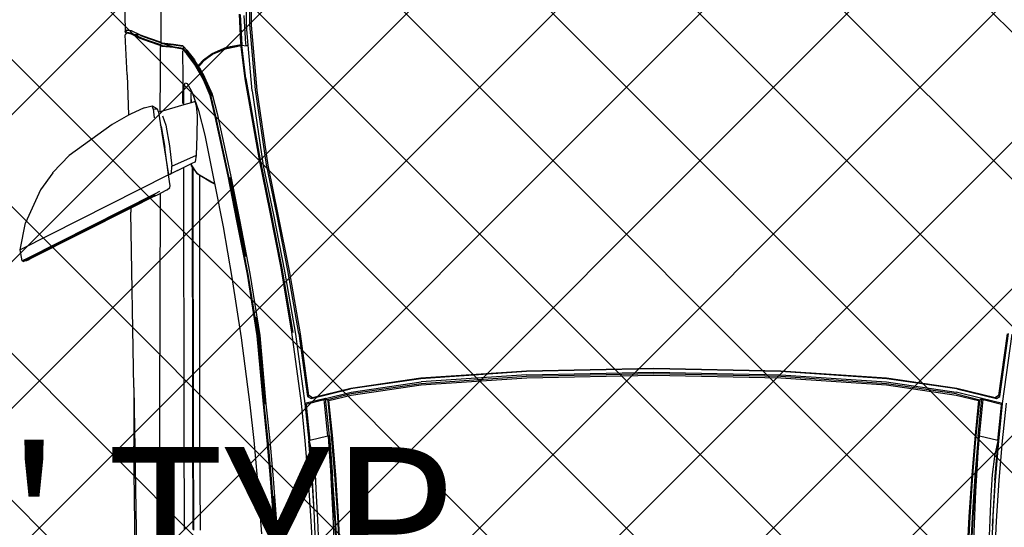
# Model space of a CAD drawing. Units: inches. Extents: x 2167 to 2589, y 1680 to 2489.
# Tile 9 of 38: x 2251 to 2299, y 1771 to 1796. Entities that reach past the tile are written whole.
import ezdxf

# ---------------------------------------------------------------- set-up
doc = ezdxf.new("R2010")
doc.units = ezdxf.units.IN
doc.header["$MEASUREMENT"] = 0
doc.layers.get('0').update_dxf_attribs({"color": 250})
for name, color, linetype, lineweight in [('A-ANNO-DIMS', 2, 'Continuous', 18), ('C-PRKG-VEHS', 8, 'Continuous', 13), ('L-PVMT-PATT', 252, 'Continuous', 13)]:
    doc.layers.add(name, color=color, linetype=linetype, lineweight=lineweight)
doc.layers.add('Edges', color=250, linetype='Continuous')
doc.styles.get("Standard").update_dxf_attribs({"font": 'arial.ttf'})
doc.dimstyles.get("Standard").update_dxf_attribs({"dimtxt": 7, "dimasz": 0.18, "dimexe": 0.18, "dimexo": 0.0625, "dimgap": 0.09, "dimtad": 0, "dimtih": 1, "dimtoh": 1, "dimdec": 1, "dimzin": 0, "dimdsep": 46, "dimlunit": 3, "dimtxsty": 'Standard', "dimcen": 0.09, "dimadec": 0, "dimazin": 0, "dimtfac": 1, "dimtdec": 1, "dimtofl": 0, "dimtmove": 0, "dimatfit": 3, "dimfxl": 1, "dimtolj": 1, "dimtzin": 0, "dimarcsym": 0})

# ---------------------------------------------------------------- blocks, each defined once
blk = doc.blocks.new('Nissan Qashqai pl')
at = {"layer": 'Edges'}
for p, q in [((9.2669, 12.5088), (9.1605, 12.5233)), ((9.1612, 12.5208), (9.2656, 12.5065)), ((9.2789, 12.5131), (9.1617, 12.5292)), ((9.2783, 12.5191), (9.3422, 12.5126)), ((9.2694, 12.5006), (9.2535, 12.4354)), ((9.2543, 12.4356), (9.2707, 12.5028)), ((9.2656, 12.5065), (9.2669, 12.5088)), ((9.2656, 12.5065), (9.2694, 12.5006)), ((9.2707, 12.5028), (9.2669, 12.5088)), ((9.2707, 12.5028), (9.2694, 12.5006)), ((9.2789, 12.5131), (9.2704, 12.4783)), ((9.2724, 12.4804), (9.2799, 12.5114)), ((9.2799, 12.5114), (9.2789, 12.5131)), ((9.3427, 12.5066), (9.2789, 12.5131)), ((9.2819, 12.5112), (9.2799, 12.5114)), ((9.2803, 12.5116), (9.2822, 12.5118)), ((9.3418, 12.5051), (9.2819, 12.5112)), ((9.3418, 12.5051), (9.3346, 12.4741)), ((9.342, 12.5059), (9.3418, 12.5051)), ((9.3687, 12.5), (9.342, 12.5059)), ((9.4087, 12.5003), (9.342, 12.5059)), ((9.3422, 12.5126), (9.4088, 12.507)), ((9.4093, 12.5011), (9.3427, 12.5066)), ((9.3992, 12.496), (9.3687, 12.5)), ((9.4087, 12.5003), (9.4688, 12.4968)), ((9.4088, 12.507), (9.4782, 12.5024)), ((9.4785, 12.4965), (9.4093, 12.5011)), ((9.4688, 12.4968), (9.4789, 12.4964)), ((9.4782, 12.5024), (9.5503, 12.4987)), ((9.2724, 12.4804), (9.2704, 12.4783)), ((9.3346, 12.4741), (9.2724, 12.4804)), ((9.4347, 12.494), (9.3992, 12.496)), ((9.4761, 12.4919), (9.4347, 12.494)), ((9.5168, 12.4903), (9.4761, 12.4919)), ((9.4789, 12.4964), (9.4785, 12.4965)), ((9.4862, 12.4961), (9.4785, 12.4965)), ((9.4789, 12.4964), (9.4862, 12.4961)), ((9.4862, 12.4961), (9.514, 12.4949)), ((9.2704, 12.4783), (9.2598, 12.4348)), ((9.2629, 12.435), (9.2726, 12.4746)), ((9.2649, 12.4348), (9.2741, 12.4725)), ((9.2726, 12.4746), (9.2704, 12.4783)), ((9.3346, 12.4718), (9.2704, 12.4783)), ((9.2746, 12.4744), (9.2726, 12.4746)), ((9.2741, 12.4725), (9.3326, 12.4666)), ((9.333, 12.4685), (9.2746, 12.4744)), ((9.3326, 12.4666), (9.4, 12.4609)), ((9.4004, 12.4629), (9.333, 12.4685)), ((9.3346, 12.4741), (9.3344, 12.4733)), ((9.3344, 12.4733), (9.4017, 12.4677)), ((9.3344, 12.4733), (9.3611, 12.4715)), ((9.3346, 12.4718), (9.4018, 12.4661)), ((9.3611, 12.4715), (9.3918, 12.4695)), ((9.3918, 12.4695), (9.4276, 12.4674)), ((9.4017, 12.4677), (9.472, 12.463)), ((9.4018, 12.4661), (9.472, 12.4614)), ((9.4276, 12.4674), (9.4694, 12.4654)), ((9.4694, 12.4654), (9.5105, 12.4637)), ((9.4, 12.4609), (9.4706, 12.4561)), ((9.4709, 12.4581), (9.4004, 12.4629)), ((9.4706, 12.4561), (9.5443, 12.4522)), ((9.5446, 12.4542), (9.4709, 12.4581)), ((9.472, 12.463), (9.5454, 12.4591)), ((9.472, 12.4614), (9.5454, 12.4576)), ((9.2535, 12.4354), (9.2362, 12.3167)), ((9.2543, 12.4356), (9.2371, 12.3169)), ((9.2426, 12.3164), (9.2598, 12.4348)), ((9.2629, 12.435), (9.2457, 12.3164)), ((9.2476, 12.3163), (9.2649, 12.4348)), ((9.2362, 12.3167), (9.2241, 12.1376)), ((9.2371, 12.3169), (9.2249, 12.1376)), ((9.2305, 12.1375), (9.2426, 12.3164)), ((9.2457, 12.3164), (9.2335, 12.1374)), ((9.2355, 12.1374), (9.2476, 12.3163)), ((9.2241, 12.1376), (9.2195, 11.9221)), ((9.2249, 12.1376), (9.2203, 11.9221)), ((9.2259, 11.9221), (9.2305, 12.1375)), ((9.2335, 12.1374), (9.2289, 11.9221)), ((9.2308, 11.9221), (9.2355, 12.1374)), ((9.2195, 11.9221), (9.2241, 11.7066)), ((9.2203, 11.9221), (9.2249, 11.7065)), ((9.2305, 11.7067), (9.2259, 11.9221)), ((9.2289, 11.9221), (9.2335, 11.7067)), ((9.2355, 11.7068), (9.2308, 11.9221)), ((9.2241, 11.7066), (9.2362, 11.5274)), ((9.2249, 11.7065), (9.2371, 11.5273)), ((9.2305, 11.7067), (9.2426, 11.5277)), ((9.2335, 11.7067), (9.2457, 11.5277)), ((9.2476, 11.5278), (9.2355, 11.7068)), ((9.2362, 11.5274), (9.2535, 11.4087)), ((9.2371, 11.5273), (9.2543, 11.4085)), ((9.2598, 11.4093), (9.2426, 11.5277)), ((9.2457, 11.5277), (9.2629, 11.4092)), ((9.2649, 11.4094), (9.2476, 11.5278)), ((9.2535, 11.4087), (9.2694, 11.3436)), ((9.2707, 11.3414), (9.2543, 11.4085)), ((9.2704, 11.3659), (9.2598, 11.4093)), ((9.2629, 11.4092), (9.2726, 11.3695)), ((9.2741, 11.3716), (9.2649, 11.4094)), ((9.4, 11.3832), (9.3326, 11.3776)), ((9.333, 11.3757), (9.4004, 11.3813)), ((9.4706, 11.388), (9.4, 11.3832)), ((9.4004, 11.3813), (9.4709, 11.3861)), ((9.472, 11.3812), (9.4017, 11.3765)), ((9.472, 11.3828), (9.4018, 11.378)), ((9.4694, 11.3788), (9.4276, 11.3767)), ((9.5105, 11.3805), (9.4694, 11.3788)), ((9.5443, 11.3919), (9.4706, 11.388)), ((9.4709, 11.3861), (9.5446, 11.39)), ((9.5454, 11.3866), (9.472, 11.3828)), ((9.472, 11.3812), (9.5454, 11.3851)), ((9.3346, 11.3724), (9.2704, 11.3659)), ((9.2704, 11.3659), (9.2726, 11.3695)), ((9.2704, 11.3659), (9.2724, 11.3637)), ((9.2704, 11.3659), (9.2789, 11.331)), ((9.3346, 11.37), (9.2724, 11.3637)), ((9.2799, 11.3328), (9.2724, 11.3637)), ((9.2726, 11.3695), (9.2746, 11.3697)), ((9.3326, 11.3776), (9.2741, 11.3716)), ((9.2746, 11.3697), (9.333, 11.3757)), ((9.4017, 11.3765), (9.3344, 11.3708)), ((9.3611, 11.3727), (9.3344, 11.3708)), ((9.3344, 11.3708), (9.3346, 11.37)), ((9.3346, 11.3724), (9.4018, 11.378)), ((9.3346, 11.37), (9.3418, 11.3391)), ((9.3918, 11.3747), (9.3611, 11.3727)), ((9.4276, 11.3767), (9.3918, 11.3747)), ((9.3687, 11.3441), (9.3992, 11.3482)), ((9.3992, 11.3482), (9.4347, 11.3502)), ((9.4605, 11.3465), (9.4087, 11.3438)), ((9.4605, 11.3465), (9.4093, 11.3431)), ((9.4347, 11.3502), (9.4761, 11.3522)), ((9.514, 11.3492), (9.4605, 11.3465)), ((9.4761, 11.3522), (9.5168, 11.3539)), ((9.5503, 11.3455), (9.4782, 11.3418)), ((9.1605, 11.3208), (9.2669, 11.3354)), ((9.2656, 11.3376), (9.1612, 11.3233)), ((9.1617, 11.315), (9.2789, 11.331)), ((9.2694, 11.3436), (9.2656, 11.3376)), ((9.2669, 11.3354), (9.2656, 11.3376)), ((9.2669, 11.3354), (9.2707, 11.3414)), ((9.2694, 11.3436), (9.2707, 11.3414)), ((9.3422, 11.3316), (9.2783, 11.3251)), ((9.2789, 11.331), (9.3427, 11.3375)), ((9.2789, 11.331), (9.2799, 11.3327)), ((9.2799, 11.3328), (9.2819, 11.333)), ((9.2799, 11.3327), (9.2799, 11.3328)), ((9.2799, 11.3327), (9.2811, 11.3325)), ((9.2819, 11.333), (9.3418, 11.3391)), ((9.3418, 11.3391), (9.342, 11.3383)), ((9.342, 11.3383), (9.3687, 11.3441)), ((9.342, 11.3383), (9.4087, 11.3438)), ((9.4088, 11.3371), (9.3422, 11.3316)), ((9.4093, 11.3431), (9.3427, 11.3375)), ((9.4782, 11.3418), (9.4088, 11.3371)), ((9.1605, 11.3208), (9.0538, 11.3023)), ((9.1612, 11.3233), (9.0546, 11.3048)), ((9.0552, 11.2965), (9.1617, 11.315)), ((9.2783, 11.3251), (9.1584, 11.3091)), ((9.0538, 11.3023), (8.9583, 11.2833)), ((9.0546, 11.3048), (8.9591, 11.2859)), ((8.9598, 11.2775), (9.0552, 11.2965)), ((9.1584, 11.3091), (9.0495, 11.2906)), ((9.0497, 11.2918), (9.1586, 11.3104)), ((8.9583, 11.2833), (8.8745, 11.266)), ((8.9591, 11.2859), (8.8754, 11.2687)), ((9.0495, 11.2906), (8.9521, 11.2715)), ((8.9522, 11.2728), (9.0497, 11.2918)), ((9.4736, 11.2793), (9.4063, 11.2743)), ((9.4064, 11.277), (9.4739, 11.282)), ((9.4727, 11.2808), (9.4362, 11.278)), ((9.4727, 11.2808), (9.4732, 11.2808)), ((9.5437, 11.2822), (9.4735, 11.2779)), ((9.5438, 11.2836), (9.4736, 11.2793)), ((9.4739, 11.282), (9.5443, 11.2863)), ((8.8745, 11.266), (8.7481, 11.2473)), ((8.8754, 11.2687), (8.7491, 11.2501)), ((8.8666, 11.2554), (8.9522, 11.2728)), ((8.9521, 11.2715), (8.8666, 11.2541)), ((8.8761, 11.2602), (8.9598, 11.2775)), ((9.1639, 11.2546), (9.2801, 11.2648)), ((9.2804, 11.262), (9.1645, 11.2518)), ((9.2804, 11.2635), (9.1668, 11.2533)), ((9.2801, 11.2648), (9.3418, 11.2713)), ((9.3418, 11.2671), (9.2803, 11.2606)), ((9.3419, 11.2685), (9.2804, 11.262)), ((9.3418, 11.2713), (9.4064, 11.277)), ((9.4062, 11.2729), (9.3418, 11.2671)), ((9.4063, 11.2743), (9.3419, 11.2685)), ((9.4735, 11.2779), (9.4062, 11.2729)), ((8.7481, 11.2473), (8.6375, 11.2376)), ((8.7491, 11.2501), (8.6386, 11.2404)), ((8.7287, 11.2307), (8.8666, 11.2554)), ((8.8666, 11.2541), (8.7292, 11.2295)), ((8.7496, 11.2416), (8.8761, 11.2602)), ((9.0591, 11.2377), (9.1639, 11.2546)), ((9.1644, 11.2503), (9.06, 11.2335)), ((9.1645, 11.2518), (9.0601, 11.235)), ((9.133, 11.2481), (9.1647, 11.2532)), ((9.2803, 11.2606), (9.1644, 11.2503)), ((9.1647, 11.2532), (9.1668, 11.2533)), ((9.3416, 11.2442), (9.4048, 11.2501)), ((9.4048, 11.2501), (9.471, 11.2554)), ((9.471, 11.2554), (9.4997, 11.2573)), ((8.6375, 11.2376), (8.5531, 11.2387)), ((8.6386, 11.2404), (8.5544, 11.2416)), ((8.6387, 11.2319), (8.555, 11.233)), ((8.6699, 11.231), (8.622, 11.228)), ((8.6721, 11.2348), (8.6387, 11.2319)), ((8.6721, 11.2312), (8.6699, 11.231)), ((8.7496, 11.2416), (8.6721, 11.2348)), ((8.6721, 11.2348), (8.6733, 11.2313)), ((8.6721, 11.2312), (8.6721, 11.2318)), ((8.6721, 11.2241), (8.6733, 11.2313)), ((8.6733, 11.2313), (8.6721, 11.2312)), ((8.7287, 11.2307), (8.6721, 11.2241)), ((8.7292, 11.2295), (8.6753, 11.2232)), ((9.0601, 11.235), (8.8941, 11.2023)), ((8.9679, 11.2201), (9.0591, 11.2377)), ((9.06, 11.2335), (8.9696, 11.2157)), ((8.9708, 11.2185), (9.03, 11.2304)), ((9.1676, 11.2229), (9.2814, 11.2377)), ((9.2814, 11.2377), (9.3416, 11.2442)), ((8.6683, 11.2226), (8.6197, 11.2201)), ((8.6203, 11.2213), (8.6721, 11.2241)), ((8.671, 11.2227), (8.6683, 11.2226)), ((8.6721, 11.2241), (8.671, 11.2227)), ((8.6716, 11.2199), (8.671, 11.2227)), ((8.6759, 11.1982), (8.6716, 11.2199)), ((8.6721, 11.2241), (8.6727, 11.2229)), ((8.6772, 11.1988), (8.6721, 11.2241)), ((8.6753, 11.2232), (8.6727, 11.2229)), ((8.6777, 11.1984), (8.6727, 11.2229)), ((8.8918, 11.205), (8.9679, 11.2201)), ((8.9696, 11.2157), (8.8942, 11.2009)), ((8.9318, 11.211), (8.9704, 11.2185)), ((8.9704, 11.2185), (8.9708, 11.2185)), ((9.0656, 11.207), (9.1676, 11.2229)), ((8.6864, 11.1736), (8.6759, 11.1982)), ((8.6875, 11.1744), (8.6772, 11.1988)), ((8.6777, 11.1984), (8.6883, 11.1737)), ((8.7881, 11.1821), (8.8918, 11.205)), ((8.8941, 11.2023), (8.7925, 11.1802)), ((8.8942, 11.2009), (8.7931, 11.1789)), ((8.8961, 11.204), (8.9318, 11.211)), ((8.9797, 11.1924), (9.0656, 11.207)), ((8.7931, 11.1789), (8.7574, 11.1704)), ((8.7575, 11.1744), (8.7881, 11.1821)), ((8.7925, 11.1802), (8.7591, 11.1723)), ((8.9087, 11.1783), (8.9797, 11.1924)), ((8.697, 11.1592), (8.6864, 11.1736)), ((8.6979, 11.1603), (8.6875, 11.1744)), ((8.6883, 11.1737), (8.6987, 11.1597)), ((8.7075, 11.1487), (8.7346, 11.1636)), ((8.7508, 11.1722), (8.7257, 11.1609)), ((8.7529, 11.17), (8.7302, 11.1602)), ((8.7574, 11.1704), (8.7312, 11.1591)), ((8.7346, 11.1636), (8.7577, 11.1732)), ((8.7346, 11.1636), (8.7491, 11.1703)), ((8.7491, 11.1703), (8.7576, 11.1743)), ((8.7508, 11.1722), (8.7491, 11.1703)), ((8.7532, 11.1733), (8.7508, 11.1722)), ((8.7529, 11.17), (8.7577, 11.1732)), ((8.757, 11.1718), (8.7529, 11.17)), ((8.7532, 11.1733), (8.7575, 11.1744)), ((8.7587, 11.1722), (8.757, 11.1718)), ((8.7575, 11.1744), (8.7576, 11.1743)), ((8.7576, 11.1743), (8.7582, 11.1734)), ((8.7577, 11.1732), (8.7582, 11.1734)), ((8.7582, 11.1734), (8.759, 11.1725)), ((8.759, 11.1725), (8.7587, 11.1722)), ((8.7591, 11.1723), (8.7587, 11.1722)), ((8.759, 11.1725), (8.7591, 11.1723)), ((8.8245, 11.1613), (8.9063, 11.1779)), ((8.8893, 11.1486), (8.9021, 11.1697)), ((8.9041, 11.1717), (8.8927, 11.1528)), ((8.9021, 11.1697), (8.9063, 11.1779)), ((8.9075, 11.1781), (8.9041, 11.1717)), ((8.9063, 11.1779), (8.9075, 11.1781)), ((8.9075, 11.1781), (8.9087, 11.1783)), ((8.6917, 11.1371), (8.7075, 11.1487)), ((8.7055, 11.1514), (8.697, 11.1592)), ((8.6987, 11.1596), (8.6979, 11.1603)), ((8.7071, 11.15), (8.6981, 11.1446)), ((8.6987, 11.1597), (8.6988, 11.1596)), ((8.6987, 11.1596), (8.6988, 11.1596)), ((8.6996, 11.1588), (8.6987, 11.1596)), ((8.6988, 11.1596), (8.6996, 11.1588)), ((8.6996, 11.1588), (8.6996, 11.1588)), ((8.7062, 11.1527), (8.6996, 11.1588)), ((8.6996, 11.1588), (8.7062, 11.1527)), ((8.7302, 11.1602), (8.7032, 11.145)), ((8.7312, 11.1591), (8.7042, 11.144)), ((8.707, 11.15), (8.7055, 11.1514)), ((8.7067, 11.1522), (8.7062, 11.1527)), ((8.7083, 11.1508), (8.7067, 11.1522)), ((8.707, 11.15), (8.7083, 11.1508)), ((8.7071, 11.15), (8.707, 11.15)), ((8.707, 11.15), (8.707, 11.15)), ((8.7083, 11.1508), (8.7071, 11.15)), ((8.7083, 11.1507), (8.7102, 11.1519)), ((8.7083, 11.1508), (8.7083, 11.1507)), ((8.7102, 11.1519), (8.7108, 11.1523)), ((8.7108, 11.1523), (8.7257, 11.1609)), ((8.7108, 11.1523), (8.7248, 11.1605)), ((8.7248, 11.1605), (8.7257, 11.1609)), ((8.7524, 11.1401), (8.7828, 11.1508)), ((8.7748, 11.1475), (8.7678, 11.1453)), ((8.7678, 11.1453), (8.7698, 11.1385)), ((8.7916, 11.1488), (8.7748, 11.1475)), ((8.7828, 11.1508), (8.8245, 11.1613)), ((8.8259, 11.1483), (8.7916, 11.1488)), ((8.8585, 11.1473), (8.8259, 11.1483)), ((8.87, 11.1455), (8.8585, 11.1473)), ((8.8771, 11.1054), (8.8585, 11.1473)), ((8.87, 11.1455), (8.8734, 11.1385)), ((8.8893, 11.1486), (8.8751, 11.1387)), ((8.881, 11.1418), (8.8893, 11.1486)), ((8.8913, 11.1506), (8.8893, 11.1486)), ((8.8927, 11.1528), (8.8913, 11.1506)), ((9.3225, 11.1531), (8.8927, 11.1528)), ((9.4936, 11.1538), (9.3225, 11.1531)), ((8.6805, 11.1309), (8.6746, 11.1253)), ((8.687, 11.131), (8.6788, 11.1237)), ((8.6805, 11.1309), (8.6884, 11.1371)), ((8.6815, 11.128), (8.6818, 11.1288)), ((8.6859, 11.132), (8.6817, 11.1282)), ((8.6817, 11.1282), (8.6818, 11.1288)), ((8.6818, 11.1288), (8.6902, 11.136)), ((8.6927, 11.1371), (8.6859, 11.132)), ((8.7042, 11.144), (8.687, 11.131)), ((8.6884, 11.1371), (8.6973, 11.144)), ((8.6884, 11.1371), (8.6917, 11.1371)), ((8.6902, 11.136), (8.6917, 11.1371)), ((8.6923, 11.1371), (8.6927, 11.1371)), ((8.7032, 11.145), (8.6927, 11.1371)), ((8.6973, 11.144), (8.698, 11.1446)), ((8.698, 11.1446), (8.6981, 11.1446)), ((8.7361, 11.1283), (8.7373, 11.1314)), ((8.7373, 11.1314), (8.7492, 11.1383)), ((8.7492, 11.1383), (8.7524, 11.1401)), ((8.7492, 11.1383), (8.7572, 11.1379)), ((8.7572, 11.1379), (8.7698, 11.1383)), ((8.7698, 11.1385), (8.7583, 11.1382)), ((8.7698, 11.1385), (8.7698, 11.1383)), ((8.7698, 11.1383), (8.7733, 11.126)), ((8.8734, 11.1385), (8.8793, 11.1261)), ((8.8734, 11.1385), (8.8768, 11.1385)), ((8.8751, 11.1387), (8.8768, 11.1385)), ((8.8768, 11.1385), (8.879, 11.1402)), ((8.879, 11.1402), (8.881, 11.1418)), ((8.879, 11.1402), (9.3198, 11.1403)), ((9.3225, 11.1421), (8.881, 11.1418)), ((9.3198, 11.1403), (9.4922, 11.1409)), ((9.4936, 11.1428), (9.3225, 11.1421)), ((8.6703, 11.1081), (8.6727, 11.1235)), ((8.6714, 11.1088), (8.6737, 11.1245)), ((8.6727, 11.1235), (8.6737, 11.1245)), ((8.6737, 11.1245), (8.6746, 11.1253)), ((8.6746, 11.1253), (8.6785, 11.1253)), ((8.6777, 11.1246), (8.6755, 11.1099)), ((8.6788, 11.1237), (8.6764, 11.1083)), ((8.6785, 11.1253), (8.6777, 11.1246)), ((8.6815, 11.128), (8.6785, 11.1253)), ((8.6817, 11.1282), (8.6815, 11.128)), ((8.6818, 11.1238), (8.7026, 11.1238)), ((8.7026, 11.1238), (8.7026, 11.1239)), ((8.7026, 11.1238), (8.7072, 11.1239)), ((8.7072, 11.1239), (8.7072, 11.1239)), ((8.7072, 11.1239), (8.7273, 11.1239)), ((8.7273, 11.1239), (8.7273, 11.124)), ((8.7273, 11.1239), (8.7354, 11.124)), ((8.7354, 11.1241), (8.7354, 11.124)), ((8.7354, 11.124), (8.742, 11.124)), ((8.7415, 11.1265), (8.7361, 11.1283)), ((8.7534, 11.1257), (8.7415, 11.1265)), ((8.742, 11.1241), (8.742, 11.124)), ((8.742, 11.124), (8.742, 11.1241)), ((8.742, 11.124), (8.742, 11.124)), ((8.742, 11.124), (8.7426, 11.124)), ((8.7426, 11.1241), (8.7426, 11.124)), ((8.7426, 11.124), (8.7433, 11.124)), ((8.7433, 11.1241), (8.7433, 11.124)), ((8.7433, 11.124), (8.7711, 11.1241)), ((8.7711, 11.1241), (8.7516, 11.1241)), ((8.7718, 11.126), (8.7534, 11.1257)), ((8.7733, 11.126), (8.7718, 11.126)), ((8.7733, 11.126), (8.7849, 11.0859)), ((9.3194, 11.1262), (8.8793, 11.1261)), ((8.8793, 11.1261), (8.8815, 11.1214)), ((8.8815, 11.1214), (8.892, 11.0998)), ((8.8815, 11.1214), (8.8895, 11.1048)), ((9.4919, 11.1269), (9.3194, 11.1262)), ((8.6684, 11.0892), (8.6703, 11.1081)), ((8.6697, 11.0922), (8.6714, 11.1088)), ((8.6698, 11.0925), (8.6755, 11.1099)), ((8.6754, 11.1089), (8.6735, 11.0898)), ((8.6764, 11.1082), (8.6744, 11.0891)), ((8.6755, 11.1099), (8.6754, 11.1089)), ((8.6764, 11.1082), (8.6764, 11.1083)), ((8.7917, 11.0895), (8.8075, 11.0955)), ((8.807, 11.0862), (8.8918, 11.0997)), ((8.8075, 11.0955), (8.8429, 11.1016)), ((8.8429, 11.1016), (8.8771, 11.1054)), ((8.8918, 11.0997), (8.8455, 11.0936)), ((8.8895, 11.1048), (8.8771, 11.1054)), ((8.8908, 11.1021), (8.8895, 11.1048)), ((8.8906, 11.1024), (8.8895, 11.1048)), ((8.8906, 11.1024), (8.8911, 11.1013)), ((8.892, 11.0998), (8.8908, 11.1021)), ((8.8911, 11.1013), (8.8919, 11.0997)), ((8.8911, 11.1013), (8.8919, 11.0998)), ((8.8919, 11.0997), (8.8911, 11.1013)), ((8.8919, 11.0997), (8.8918, 11.0997)), ((8.8918, 11.0997), (9.0186, 10.8486)), ((8.892, 11.0998), (8.8919, 11.0998)), ((8.8919, 11.0998), (8.8919, 11.0997)), ((8.8919, 11.0997), (8.8919, 11.0997)), ((8.9106, 11.1029), (8.892, 11.0998)), ((8.892, 11.0998), (8.892, 11.0998)), ((8.9131, 11.102), (8.9106, 11.1029)), ((8.9171, 11.0978), (8.9131, 11.102)), ((8.9171, 11.0978), (8.917, 11.0974)), ((8.9171, 11.0978), (8.9233, 11.0855)), ((8.5326, 11.0874), (8.6675, 11.0866)), ((8.6606, 11.0674), (8.6667, 11.0857)), ((8.6616, 11.0683), (8.6675, 11.0862)), ((8.6718, 11.0868), (8.6657, 11.0684)), ((8.6667, 11.0857), (8.6675, 11.0862)), ((8.6728, 11.0858), (8.6667, 11.0675)), ((8.6674, 11.0864), (8.6675, 11.0865)), ((8.6675, 11.0865), (8.6675, 11.0866)), ((8.6676, 11.0866), (8.6675, 11.0866)), ((8.6675, 11.0862), (8.6679, 11.0864)), ((8.6676, 11.0864), (8.6677, 11.0866)), ((8.6677, 11.0866), (8.6676, 11.0866)), ((8.6682, 11.0866), (8.6677, 11.0866)), ((8.6679, 11.0864), (8.6682, 11.0866)), ((8.6682, 11.087), (8.6684, 11.0888)), ((8.6692, 11.0876), (8.6682, 11.0866)), ((8.6682, 11.087), (8.6692, 11.0876)), ((8.6682, 11.0866), (8.6682, 11.087)), ((8.6684, 11.0888), (8.6684, 11.0892)), ((8.6684, 11.0888), (8.6685, 11.089)), ((8.6692, 11.0876), (8.6697, 11.0922)), ((8.6697, 11.0922), (8.6698, 11.0925)), ((8.6729, 11.0874), (8.6718, 11.0868)), ((8.674, 11.0864), (8.6728, 11.0858)), ((8.6733, 11.0875), (8.6729, 11.0874)), ((8.6735, 11.0898), (8.6733, 11.0875)), ((8.6742, 11.0866), (8.674, 11.0864)), ((8.6744, 11.0891), (8.6742, 11.0866)), ((8.6744, 11.0866), (8.6742, 11.0866)), ((8.6742, 11.0858), (8.6743, 11.086)), ((8.6744, 11.0864), (8.6744, 11.0866)), ((8.6773, 11.0865), (8.6744, 11.0866)), ((8.6791, 11.0864), (8.677, 11.0864)), ((8.6791, 11.0865), (8.6773, 11.0865)), ((8.6791, 11.0865), (8.6791, 11.0864)), ((8.6878, 11.0864), (8.6791, 11.0865)), ((8.7205, 11.0863), (8.6791, 11.0864)), ((8.6878, 11.0864), (8.6791, 11.0864)), ((8.6878, 11.0865), (8.6878, 11.0864)), ((8.6911, 11.0864), (8.6878, 11.0864)), ((8.7205, 11.0863), (8.6911, 11.0864)), ((8.7849, 11.0859), (8.7205, 11.0863)), ((8.7779, 11.0773), (8.7807, 11.0812)), ((8.7798, 11.0739), (8.7807, 11.0812)), ((8.7849, 11.0827), (8.7807, 11.0812)), ((8.7849, 11.0859), (8.7856, 11.0834)), ((8.7849, 11.0827), (8.7858, 11.0828)), ((8.7858, 11.0828), (8.7856, 11.0834)), ((8.7858, 11.0828), (8.807, 11.0862)), ((8.8102, 11.0874), (8.807, 11.0862)), ((8.8102, 11.0874), (8.8455, 11.0936)), ((8.9232, 11.0779), (8.9194, 11.0854)), ((8.9233, 11.0855), (9.2886, 11.0848)), ((8.925, 11.0821), (8.9233, 11.0855)), ((8.928, 11.0762), (8.925, 11.0821)), ((9.2886, 11.0848), (9.4673, 11.0852)), ((9.4673, 11.0852), (9.6358, 11.0866)), ((8.6546, 11.0516), (8.6606, 11.0674)), ((8.6556, 11.0524), (8.6616, 11.0683)), ((8.6657, 11.0684), (8.6598, 11.0529)), ((8.6667, 11.0675), (8.6608, 11.0521)), ((8.7751, 11.0723), (8.7779, 11.0773)), ((8.7798, 11.0739), (8.7751, 11.0723)), ((8.7785, 11.0587), (8.7751, 11.0723)), ((8.7798, 11.0739), (8.7954, 11.0758)), ((9.0333, 10.8597), (8.9232, 11.0779)), ((9.0386, 10.8534), (8.9254, 11.0778)), ((8.928, 11.0762), (8.9483, 11.0359)), ((8.6472, 11.0366), (8.6546, 11.0516)), ((8.6482, 11.0375), (8.655, 11.0513)), ((8.6608, 11.0521), (8.6534, 11.0369)), ((8.6598, 11.0529), (8.655, 11.0432)), ((8.655, 11.0513), (8.6556, 11.0524)), ((8.655, 11.0513), (8.655, 11.0432)), ((8.7785, 11.0587), (8.7891, 11.0353)), ((9.2517, 11.0411), (9.5372, 11.0459)), ((9.641, 11.045), (9.351, 11.0411)), ((8.646, 11.0289), (8.6468, 11.0337)), ((8.6489, 11.0263), (8.646, 11.0289)), ((8.6468, 11.0337), (8.6472, 11.0366)), ((8.647, 11.03), (8.6468, 11.0337)), ((8.647, 11.03), (8.6482, 11.0375)), ((8.6498, 11.0273), (8.647, 11.03)), ((8.6527, 11.0286), (8.6489, 11.0263)), ((8.6524, 11.0289), (8.6498, 11.0273)), ((8.6524, 11.0378), (8.651, 11.0302)), ((8.651, 11.0302), (8.652, 11.0292)), ((8.6534, 11.0369), (8.652, 11.0292)), ((8.652, 11.0292), (8.6524, 11.0289)), ((8.655, 11.0432), (8.6524, 11.0378)), ((8.6524, 11.0289), (8.6527, 11.0286)), ((8.6527, 11.0286), (8.6537, 11.0275)), ((8.7222, 11.0298), (8.6547, 11.0265)), ((8.7222, 11.0298), (8.7908, 11.0322)), ((8.7891, 11.0353), (8.7908, 11.0322)), ((8.7908, 11.0322), (8.8066, 11.0041)), ((8.9483, 11.0359), (8.9552, 11.0361)), ((8.9483, 11.0359), (9.0343, 10.8656)), ((9.2517, 11.0411), (8.9552, 11.0361)), ((9.2517, 11.0411), (9.351, 11.0411)), ((8.5838, 11.0251), (8.6489, 11.0263)), ((8.6547, 11.0265), (8.6537, 11.0275)), ((8.6537, 11.0275), (8.6537, 11.0275)), ((8.8066, 11.0041), (8.8591, 10.9315)), ((8.8591, 10.9315), (8.8879, 10.9041)), ((8.8885, 10.9037), (8.8879, 10.9041)), ((8.8885, 10.9037), (8.9173, 10.8831)), ((8.9173, 10.8831), (8.9731, 10.8577)), ((9.0343, 10.8656), (9.0347, 10.8648)), ((9.0347, 10.8648), (9.0362, 10.8619)), ((9.0362, 10.8619), (9.037, 10.8603)), ((9.0186, 10.8486), (8.9731, 10.8577)), ((9.0374, 10.8517), (9.0186, 10.8486)), ((9.0356, 10.8553), (9.0333, 10.8597)), ((9.0356, 10.8553), (9.0374, 10.8517)), ((9.0371, 10.8601), (9.037, 10.8603)), ((9.0371, 10.8601), (9.0376, 10.8591)), ((9.0376, 10.8591), (9.0371, 10.8595)), ((9.0386, 10.8534), (9.0374, 10.8517)), ((9.0376, 10.8591), (9.0386, 10.8534))]:
    blk.add_line(p, q, dxfattribs=at)
blk = doc.blocks.new('car')
blk.add_blockref('Nissan Qashqai pl', (-9.7433, -11.9151))
blk = doc.blocks.new('carr')
blk.add_blockref('car', (0.5124, -0.007))
blk = doc.blocks.new('*D45')
at = {"layer": 'A-ANNO-DIMS', "color": 0, "lineweight": -2, "transparency": 16777216}
for p, q in [((2251.156, 1833.955), (2232.359, 1833.955)), ((2232.539, 1833.775), (2232.539, 1775.399)), ((2232.539, 1709.605), (2232.539, 1767.981)), ((2251.156, 1709.425), (2232.359, 1709.425))]:
    blk.add_line(p, q, dxfattribs=at)
at = {"layer": 'A-ANNO-DIMS', "color": 0, "transparency": 16777216}
for points in [[(2232.509, 1833.775), (2232.569, 1833.775), (2232.539, 1833.955)], [(2232.509, 1709.605), (2232.569, 1709.605), (2232.539, 1709.425)]]:
    blk.add_solid(points, dxfattribs=at)
at = {"layer": 'Defpoints', "color": 0, "transparency": 16777216}
for p in [(2251.218, 1833.955), (2232.539, 1709.425), (2251.218, 1709.425)]:
    blk.add_point(p, dxfattribs=at)
at = {"layer": 'A-ANNO-DIMS', "color": 0, "transparency": 16777216, "insert": (2232.539, 1771.69), "char_height": 7, "attachment_point": 5}
blk.add_mtext('\\A1;CAR 10\'-4 1/2" TYP.', dxfattribs=at)

msp = doc.modelspace()

# ---------------------------------------------------------------- hatches: boundary and pattern name
at = {"layer": 'L-PVMT-PATT'}
h = msp.add_hatch(dxfattribs=at)
h.set_pattern_fill('ANSI37', color=256, scale=40)
h.paths.add_polyline_path([(2417.548, 1783.695), (2417.548, 1846.042), (2239.361, 1846.042), (2239.361, 1687.695), (2369.843, 1687.695), (2369.843, 1696.695), (2375.607, 1696.695), (2416.107, 1696.695), (2417.548, 1696.695)])

# ---------------------------------------------------------------- block references
at = {"layer": 'C-PRKG-VEHS', "xscale": 28.42784210623918, "yscale": 28.42784210623918, "zscale": 28.42784210623918, "rotation": 270}
msp.add_blockref('carr', (2281.736, 1778.659), dxfattribs=at)

# ---------------------------------------------------------------- dimensions: what is measured, and where the dimension line sits
at = {"layer": 'A-ANNO-DIMS'}
dim = msp.add_linear_dim(base=(2232.539, 1709.425), p1=(2251.218, 1833.955), p2=(2251.218, 1709.425), angle=270, text='CAR <> TYP.', dimstyle='Standard', override={"dimdec": 1, "dimlfac": 1, "dimrnd": 0, "dimzin": 1, "dimdsep": 46, "dimlunit": 4, "dimfrac": 2}, dxfattribs=at)
dim.commit()
dim.dimension.update_dxf_attribs({"geometry": '*D45', "text_midpoint": (2232.539, 1771.69)})

doc.saveas('drawing.dxf')
